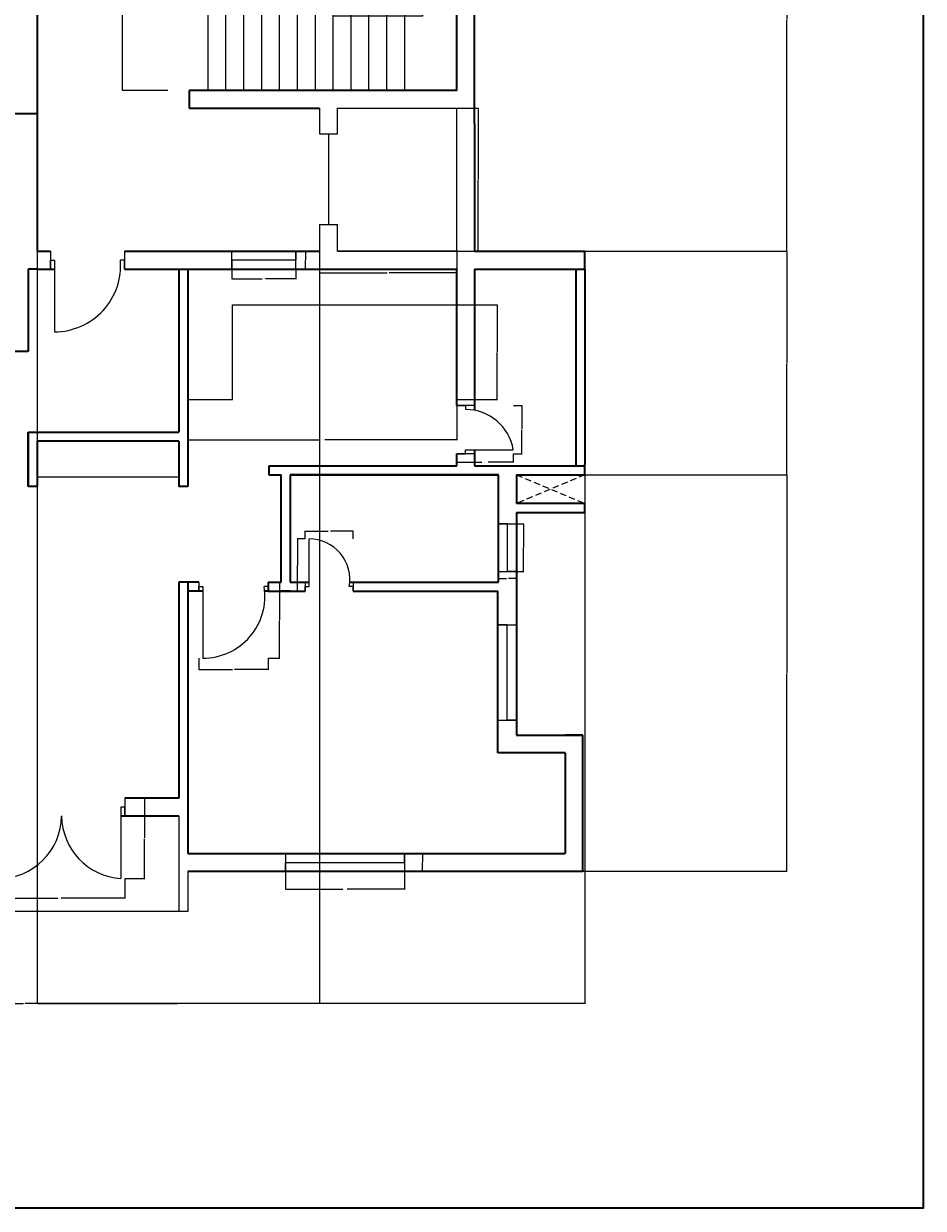
# Model space of a CAD drawing. Units: inches. Extents: x 2296 to 3812, y -1531 to 2564.
# Tile 7 of 10: x 3359 to 3812, y 1124 to 1720. Entities that reach past the tile are written whole.
import ezdxf

# ---------------------------------------------------------------- set-up
doc = ezdxf.new("R2010")
doc.units = ezdxf.units.IN
doc.linetypes.add('HIDDEN2', pattern=[4.7625, 3.175, -1.5875])
for name, color, linetype, lineweight in [('A-ANNO-DIMS', 2, 'Continuous', 18), ('A-ANNO-TTLB', 7, 'Continuous', 35), ('A-DOOR', 3, 'Continuous', 18), ('A-EQPM-ELEV', 7, 'Continuous', 25), ('A-FLOR-CASE', 8, 'Continuous', 18), ('A-FLOR-HRAL', 7, 'Continuous', 25), ('A-FLOR-STRS', 7, 'Continuous', 18), ('A-GLAZ', 4, 'Continuous', 18), ('A-WALL', 7, 'Continuous', 35), ('A-WALL-HIDN', 8, 'HIDDEN2', 18)]:
    doc.layers.add(name, color=color, linetype=linetype, lineweight=lineweight)
doc.styles.get("Standard").update_dxf_attribs({"font": 'arial.ttf'})
doc.dimstyles.get("Standard").update_dxf_attribs({"dimtxt": 0.18, "dimasz": 0.18, "dimexe": 0.18, "dimexo": 0.0625, "dimgap": 0.09, "dimtad": 0, "dimtih": 1, "dimtoh": 1, "dimdec": 4, "dimzin": 0, "dimdsep": 46, "dimtxsty": 'Standard', "dimcen": 0.09, "dimadec": 0, "dimazin": 0, "dimtfac": 1, "dimtdec": 4, "dimtofl": 0, "dimtmove": 0, "dimatfit": 3, "dimfxl": 1, "dimtolj": 1, "dimtzin": 0, "dimarcsym": 0})

# ---------------------------------------------------------------- blocks, each defined once
blk = doc.blocks.new('DOOR-ENTRY-36-S')
for p, q in [((0, 40.5), (0, 31.5)), ((0, 31.5), (0, 36)), ((0, 36), (2, 36)), ((2, 36), (2, 0)), ((37.2, 36), (35.2, 36)), ((37.2, 40.5), (37.2, 31.5)), ((37.2, 31.5), (37.2, 36))]:
    blk.add_line(p, q)
blk.add_arc((2, 33.31), 33.31, 270, 4.6283)
blk = doc.blocks.new('DOOR-BEDROOM-36-SE')
for p, q in [((0, 38.25), (0, 33.75)), ((0, 33.75), (0, 36)), ((0, 36), (2, 36)), ((2, 36), (2, 0)), ((34.88, 36), (32.88, 36))]:
    blk.add_line(p, q)
blk.add_arc((2, 31.24), 31.24, 270, 8.75969)
blk = doc.blocks.new('DOOR-BATH-24-SE')
for p, q in [((2, 2.25), (2, 26.25)), ((0, 4.5), (0, 0)), ((0, 0), (0, 2.25)), ((0, 2.25), (2, 2.25)), ((24.15, 2.25), (22.15, 2.25)), ((24.15, 4.5), (24.15, 0)), ((24.15, 0), (24.15, 2.25))]:
    blk.add_line(p, q)
blk.add_arc((2, 5.79), 20.46, 350.03773, 90)
blk = doc.blocks.new('DOOR-BALCONY-PAIR-S')
for p, q in [((0, 40.5), (0, 31.5)), ((0, 31.5), (0, 36)), ((0, 36), (2, 36)), ((2, 36), (2, 0)), ((65.68, 36), (63.68, 36)), ((63.68, 36), (63.68, 0)), ((65.68, 40.5), (65.68, 31.5)), ((65.68, 31.5), (65.68, 36))]:
    blk.add_line(p, q)
for centre, radius, start, end in [((2, 31.87), 31.87, 270, 359.32793), ((65.8, 31.86), 31.93, 180.64039, 266.18908)]:
    blk.add_arc(centre, radius, start, end)
blk = doc.blocks.new('DOOR-SERVICE-24-SE')
for p, q in [((9, 24.24), (0, 24.24)), ((0, 24.24), (4.5, 24.24)), ((4.5, 24.24), (4.5, 22.24)), ((9, 0), (0, 0)), ((0, 0), (4.5, 0)), ((4.5, 0), (4.5, 2)), ((4.5, 2), (28.5, 2))]:
    blk.add_line(p, q)
blk.add_arc((4.5, -2.11), 24.35, 9.71884, 90)
blk = doc.blocks.new('WIN-24-BATH')
for p, q in [((4.5, 24), (0, 24)), ((0, 24), (9, 24)), ((4.5, 0), (4.5, 24)), ((0, 0), (9, 0)), ((9, 0), (4.5, 0))]:
    blk.add_line(p, q)
blk = doc.blocks.new('WIN-48-BEDROOM-SE')
for p, q in [((4.71, 48), (0, 48)), ((0, 48), (9.41, 48)), ((4.71, 0), (4.71, 48)), ((0, 0), (9.41, 0)), ((9.41, 0), (4.71, 0))]:
    blk.add_line(p, q)
blk = doc.blocks.new('WIN-60-SILL')
for p, q in [((0, 9), (0, 0)), ((60, 4.5), (60, 9)), ((60, 9), (60, 0)), ((0, 0), (0, 4.5)), ((0, 4.5), (60, 4.5))]:
    blk.add_line(p, q)
blk = doc.blocks.new('WIN-32-KITCHEN')
for p, q in [((0, 9), (0, 0)), ((32.18, 4.5), (32.18, 9)), ((32.18, 9), (32.18, 0)), ((0, 0), (0, 4.5)), ((0, 4.5), (32.18, 4.5))]:
    blk.add_line(p, q)
blk = doc.blocks.new('STAIR-DOGLEG')
for p, q in [((20.27, 0), (20.27, 152.06)), ((29.27, 0), (29.27, 152.06)), ((38.27, 0), (38.27, 152.06)), ((47.27, 0), (47.27, 152.06)), ((56.27, 0), (56.27, 152.06)), ((65.27, 0), (65.27, 152.06)), ((74.27, 0), (74.27, 152.06)), ((83.27, 0), (83.27, 152.06)), ((92.27, 0), (92.27, 152.06)), ((101.27, 0), (101.27, 152.06)), ((110.27, 0), (110.27, 152.06)), ((119.27, 0), (119.27, 152.06)), ((0, 107.85), (128.27, 107.85)), ((128.27, 107.85), (128.27, 37.4)), ((20.27, 76.03), (119.27, 76.03)), ((128.27, 37.4), (83.27, 37.4))]:
    blk.add_line(p, q)
blk = doc.blocks.new('COUNTER-KITCHEN-S')
for p, q in [((22.51, 0), (22.51, 47.52)), ((22.51, 47.52), (135.34, 47.52)), ((0, 0), (0, 0)), ((0, 0), (22.51, 0))]:
    blk.add_line(p, q)
blk = doc.blocks.new('LIFT-SHAFT-60x72')
for p, q in [((0, 72), (0, 59.12)), ((9, 72), (69, 72)), ((9, 59.12), (9, 72)), ((69, 0), (69, 72)), ((0, 59.12), (9, 59.12)), ((4.5, 59.12), (4.5, 13.58)), ((0, 13.58), (9, 13.58)), ((0, 13.58), (0, 0)), ((9, 0), (9, 13.58)), ((69, 0), (9, 0)), ((9, 0), (69, 0))]:
    blk.add_line(p, q)
blk = doc.blocks.new('*D49')
at = {"layer": 'A-ANNO-DIMS', "color": 0, "lineweight": -2, "transparency": 16777216}
for p, q in [((3431.99, 1838.66), (3409.07, 1838.66)), ((3409.25, 1838.48), (3409.25, 1762.81)), ((3409.25, 1686.78), (3409.25, 1762.45)), ((3431.99, 1686.6), (3409.07, 1686.6))]:
    blk.add_line(p, q, dxfattribs=at)
at = {"layer": 'A-ANNO-DIMS', "color": 0, "transparency": 16777216}
for points in [[(3409.22, 1838.48), (3409.28, 1838.48), (3409.25, 1838.66)], [(3409.22, 1686.78), (3409.28, 1686.78), (3409.25, 1686.6)]]:
    blk.add_solid(points, dxfattribs=at)
at = {"layer": 'Defpoints', "color": 0, "transparency": 16777216}
for p in [(3409.25, 1838.66), (3432.06, 1838.66), (3432.06, 1686.6)]:
    blk.add_point(p, dxfattribs=at)
at = {"layer": 'A-ANNO-DIMS', "color": 0, "transparency": 16777216, "insert": (3409.25, 1762.63), "char_height": 0.18, "attachment_point": 5}
blk.add_mtext('\\A1;STAIR 152 TYP.', dxfattribs=at)
blk = doc.blocks.new('*D51')
at = {"layer": 'A-ANNO-DIMS', "color": 0, "lineweight": -2, "transparency": 16777216}
for p, q in [((3577.56, 1677.6), (3588.47, 1677.6)), ((3588.29, 1677.42), (3588.29, 1641.78)), ((3588.29, 1605.78), (3588.29, 1641.42)), ((3577.56, 1605.6), (3588.47, 1605.6))]:
    blk.add_line(p, q, dxfattribs=at)
at = {"layer": 'A-ANNO-DIMS', "color": 0, "transparency": 16777216}
for points in [[(3588.26, 1677.42), (3588.32, 1677.42), (3588.29, 1677.6)], [(3588.26, 1605.78), (3588.32, 1605.78), (3588.29, 1605.6)]]:
    blk.add_solid(points, dxfattribs=at)
at = {"layer": 'Defpoints', "color": 0, "transparency": 16777216}
for p in [(3577.49, 1677.6), (3588.29, 1677.6), (3577.49, 1605.6)]:
    blk.add_point(p, dxfattribs=at)
at = {"layer": 'A-ANNO-DIMS', "color": 0, "transparency": 16777216, "insert": (3588.29, 1641.6), "char_height": 0.18, "attachment_point": 5}
blk.add_mtext('\\A1;LIFT 72 TYP.', dxfattribs=at)
blk = doc.blocks.new('*D52')
at = {"layer": 'A-ANNO-DIMS', "color": 0, "lineweight": -2, "transparency": 16777216}
for p, q in [((3508.49, 1605.54), (3508.49, 1594.62)), ((3577.49, 1605.54), (3577.49, 1594.62)), ((3508.67, 1594.8), (3542.47, 1594.8)), ((3577.31, 1594.8), (3543.52, 1594.8))]:
    blk.add_line(p, q, dxfattribs=at)
at = {"layer": 'A-ANNO-DIMS', "color": 0, "transparency": 16777216}
for points in [[(3508.67, 1594.83), (3508.67, 1594.77), (3508.49, 1594.8)], [(3577.31, 1594.83), (3577.31, 1594.77), (3577.49, 1594.8)]]:
    blk.add_solid(points, dxfattribs=at)
at = {"layer": 'Defpoints', "color": 0, "transparency": 16777216}
for p in [(3508.49, 1605.6), (3577.49, 1605.6), (3577.49, 1594.8)]:
    blk.add_point(p, dxfattribs=at)
at = {"layer": 'A-ANNO-DIMS', "color": 0, "transparency": 16777216, "insert": (3542.99, 1594.8), "char_height": 0.18, "attachment_point": 5}
blk.add_mtext('\\A1;69 TYP.', dxfattribs=at)
blk = doc.blocks.new('*D55')
at = {"layer": 'A-ANNO-DIMS', "color": 0, "lineweight": -2, "transparency": 16777216}
for p, q in [((3442.16, 1531.04), (3442.16, 1510.62)), ((3577.49, 1531.04), (3577.49, 1510.62)), ((3442.34, 1510.8), (3508.57, 1510.8)), ((3577.31, 1510.8), (3511.08, 1510.8))]:
    blk.add_line(p, q, dxfattribs=at)
at = {"layer": 'A-ANNO-DIMS', "color": 0, "transparency": 16777216}
for points in [[(3442.34, 1510.83), (3442.34, 1510.77), (3442.16, 1510.8)], [(3577.31, 1510.83), (3577.31, 1510.77), (3577.49, 1510.8)]]:
    blk.add_solid(points, dxfattribs=at)
at = {"layer": 'Defpoints', "color": 0, "transparency": 16777216}
for p in [(3442.16, 1531.1), (3577.49, 1531.1), (3577.49, 1510.8)]:
    blk.add_point(p, dxfattribs=at)
at = {"layer": 'A-ANNO-DIMS', "color": 0, "transparency": 16777216, "insert": (3509.83, 1510.8), "char_height": 0.18, "attachment_point": 5}
blk.add_mtext('\\A1;COUNTER 135 TYP.', dxfattribs=at)
blk = doc.blocks.new('*D56')
at = {"layer": 'A-ANNO-DIMS', "color": 0, "lineweight": -2, "transparency": 16777216}
for p, q in [((3577.56, 1578.62), (3597.97, 1578.62)), ((3597.79, 1578.44), (3597.79, 1555.04)), ((3597.79, 1531.28), (3597.79, 1554.68)), ((3577.56, 1531.1), (3597.97, 1531.1))]:
    blk.add_line(p, q, dxfattribs=at)
at = {"layer": 'A-ANNO-DIMS', "color": 0, "transparency": 16777216}
for points in [[(3597.76, 1578.44), (3597.82, 1578.44), (3597.79, 1578.62)], [(3597.76, 1531.28), (3597.82, 1531.28), (3597.79, 1531.1)]]:
    blk.add_solid(points, dxfattribs=at)
at = {"layer": 'Defpoints', "color": 0, "transparency": 16777216}
for p in [(3577.49, 1578.62), (3597.79, 1578.62), (3577.49, 1531.1)]:
    blk.add_point(p, dxfattribs=at)
at = {"layer": 'A-ANNO-DIMS', "color": 0, "transparency": 16777216, "insert": (3597.79, 1554.86), "char_height": 0.18, "attachment_point": 5}
blk.add_mtext('\\A1;48 TYP.', dxfattribs=at)
blk = doc.blocks.new('*D79')
at = {"layer": 'A-ANNO-DIMS', "color": 0, "lineweight": -2, "transparency": 16777216}
for p, q in [((3482.65, 1439.1), (3488.51, 1439.1)), ((3488.33, 1438.92), (3488.33, 1420.16)), ((3488.33, 1401.03), (3488.33, 1419.79)), ((3482.65, 1400.85), (3488.51, 1400.85))]:
    blk.add_line(p, q, dxfattribs=at)
at = {"layer": 'A-ANNO-DIMS', "color": 0, "transparency": 16777216}
for points in [[(3488.3, 1438.92), (3488.36, 1438.92), (3488.33, 1439.1)], [(3488.3, 1401.03), (3488.36, 1401.03), (3488.33, 1400.85)]]:
    blk.add_solid(points, dxfattribs=at)
at = {"layer": 'Defpoints', "color": 0, "transparency": 16777216}
for p in [(3482.59, 1439.1), (3488.33, 1439.1), (3482.59, 1400.85)]:
    blk.add_point(p, dxfattribs=at)
at = {"layer": 'A-ANNO-DIMS', "color": 0, "transparency": 16777216, "insert": (3488.33, 1419.98), "char_height": 0.18, "attachment_point": 5}
blk.add_mtext('\\A1;DOOR 38 TYP.', dxfattribs=at)
blk = doc.blocks.new('*D80')
at = {"layer": 'A-ANNO-DIMS', "color": 0, "lineweight": -2, "transparency": 16777216}
for p, q in [((3447.71, 1400.79), (3447.71, 1394.93)), ((3447.89, 1395.11), (3464.63, 1395.11)), ((3482.41, 1395.11), (3465.68, 1395.11)), ((3482.59, 1400.79), (3482.59, 1394.93))]:
    blk.add_line(p, q, dxfattribs=at)
at = {"layer": 'A-ANNO-DIMS', "color": 0, "transparency": 16777216}
for points in [[(3447.89, 1395.14), (3447.89, 1395.08), (3447.71, 1395.11)], [(3482.41, 1395.14), (3482.41, 1395.08), (3482.59, 1395.11)]]:
    blk.add_solid(points, dxfattribs=at)
at = {"layer": 'Defpoints', "color": 0, "transparency": 16777216}
for p in [(3447.71, 1400.85), (3482.59, 1400.85), (3482.59, 1395.11)]:
    blk.add_point(p, dxfattribs=at)
at = {"layer": 'A-ANNO-DIMS', "color": 0, "transparency": 16777216, "insert": (3465.15, 1395.11), "char_height": 0.18, "attachment_point": 5}
blk.add_mtext('\\A1;35 TYP.', dxfattribs=at)
blk = doc.blocks.new('*D81')
at = {"layer": 'A-ANNO-DIMS', "color": 0, "lineweight": -2, "transparency": 16777216}
for p, q in [((3501.21, 1460.85), (3497.15, 1460.85)), ((3497.33, 1460.67), (3497.33, 1447.91)), ((3497.33, 1434.78), (3497.33, 1447.54)), ((3501.21, 1434.6), (3497.15, 1434.6))]:
    blk.add_line(p, q, dxfattribs=at)
at = {"layer": 'A-ANNO-DIMS', "color": 0, "transparency": 16777216}
for points in [[(3497.3, 1460.67), (3497.36, 1460.67), (3497.33, 1460.85)], [(3497.3, 1434.78), (3497.36, 1434.78), (3497.33, 1434.6)]]:
    blk.add_solid(points, dxfattribs=at)
at = {"layer": 'Defpoints', "color": 0, "transparency": 16777216}
for p in [(3497.33, 1460.85), (3501.27, 1460.85), (3501.27, 1434.6)]:
    blk.add_point(p, dxfattribs=at)
at = {"layer": 'A-ANNO-DIMS', "color": 0, "transparency": 16777216, "insert": (3497.33, 1447.73), "char_height": 0.18, "attachment_point": 5}
blk.add_mtext('\\A1;BATH DOOR 26 TYP.', dxfattribs=at)
blk = doc.blocks.new('*D82')
at = {"layer": 'A-ANNO-DIMS', "color": 0, "lineweight": -2, "transparency": 16777216}
for p, q in [((3501.27, 1460.91), (3501.27, 1464.97)), ((3501.45, 1464.79), (3512.82, 1464.79)), ((3525.24, 1464.79), (3513.88, 1464.79)), ((3525.42, 1460.91), (3525.42, 1464.97))]:
    blk.add_line(p, q, dxfattribs=at)
at = {"layer": 'A-ANNO-DIMS', "color": 0, "transparency": 16777216}
for points in [[(3501.45, 1464.82), (3501.45, 1464.76), (3501.27, 1464.79)], [(3525.24, 1464.82), (3525.24, 1464.76), (3525.42, 1464.79)]]:
    blk.add_solid(points, dxfattribs=at)
at = {"layer": 'Defpoints', "color": 0, "transparency": 16777216}
for p in [(3501.27, 1460.85), (3525.42, 1464.79), (3525.42, 1460.85)]:
    blk.add_point(p, dxfattribs=at)
at = {"layer": 'A-ANNO-DIMS', "color": 0, "transparency": 16777216, "insert": (3513.35, 1464.79), "char_height": 0.18, "attachment_point": 5}
blk.add_mtext('\\A1;24 TYP.', dxfattribs=at)
blk = doc.blocks.new('*D87')
at = {"layer": 'A-ANNO-DIMS', "color": 0, "lineweight": -2, "transparency": 16777216}
for p, q in [((3344.71, 1289.87), (3344.71, 1279.9)), ((3410.39, 1289.87), (3410.39, 1279.9)), ((3344.89, 1280.08), (3376.7, 1280.08)), ((3410.21, 1280.08), (3378.4, 1280.08))]:
    blk.add_line(p, q, dxfattribs=at)
at = {"layer": 'A-ANNO-DIMS', "color": 0, "transparency": 16777216}
for points in [[(3344.89, 1280.11), (3344.89, 1280.05), (3344.71, 1280.08)], [(3410.21, 1280.11), (3410.21, 1280.05), (3410.39, 1280.08)]]:
    blk.add_solid(points, dxfattribs=at)
at = {"layer": 'Defpoints', "color": 0, "transparency": 16777216}
for p in [(3344.71, 1289.93), (3410.39, 1289.93), (3410.39, 1280.08)]:
    blk.add_point(p, dxfattribs=at)
at = {"layer": 'A-ANNO-DIMS', "color": 0, "transparency": 16777216, "insert": (3377.55, 1280.08), "char_height": 0.18, "attachment_point": 5}
blk.add_mtext('\\A1;PAIR 66 TYP.', dxfattribs=at)
blk = doc.blocks.new('*D88')
at = {"layer": 'A-ANNO-DIMS', "color": 0, "lineweight": -2, "transparency": 16777216}
for p, q in [((3410.45, 1330.43), (3420.42, 1330.43)), ((3420.24, 1330.25), (3420.24, 1310.36)), ((3420.24, 1290.11), (3420.24, 1310)), ((3410.45, 1289.93), (3420.42, 1289.93))]:
    blk.add_line(p, q, dxfattribs=at)
at = {"layer": 'A-ANNO-DIMS', "color": 0, "transparency": 16777216}
for points in [[(3420.21, 1330.25), (3420.27, 1330.25), (3420.24, 1330.43)], [(3420.21, 1290.11), (3420.27, 1290.11), (3420.24, 1289.93)]]:
    blk.add_solid(points, dxfattribs=at)
at = {"layer": 'Defpoints', "color": 0, "transparency": 16777216}
for p in [(3410.39, 1330.43), (3420.24, 1330.43), (3410.39, 1289.93)]:
    blk.add_point(p, dxfattribs=at)
at = {"layer": 'A-ANNO-DIMS', "color": 0, "transparency": 16777216, "insert": (3420.24, 1310.18), "char_height": 0.18, "attachment_point": 5}
blk.add_mtext('\\A1;41 TYP.', dxfattribs=at)
blk = doc.blocks.new('*D91')
at = {"layer": 'A-ANNO-DIMS', "color": 0, "lineweight": -2, "transparency": 16777216}
for p, q in [((3577.49, 1503.68), (3577.49, 1499.29)), ((3605.99, 1503.68), (3605.99, 1499.29)), ((3577.67, 1499.47), (3590.22, 1499.47)), ((3605.81, 1499.47), (3593.27, 1499.47))]:
    blk.add_line(p, q, dxfattribs=at)
at = {"layer": 'A-ANNO-DIMS', "color": 0, "transparency": 16777216}
for points in [[(3577.67, 1499.5), (3577.67, 1499.44), (3577.49, 1499.47)], [(3605.81, 1499.5), (3605.81, 1499.44), (3605.99, 1499.47)]]:
    blk.add_solid(points, dxfattribs=at)
at = {"layer": 'Defpoints', "color": 0, "transparency": 16777216}
for p in [(3577.49, 1503.74), (3605.99, 1503.74), (3605.99, 1499.47)]:
    blk.add_point(p, dxfattribs=at)
at = {"layer": 'A-ANNO-DIMS', "color": 0, "transparency": 16777216, "insert": (3591.74, 1499.47), "char_height": 0.18, "attachment_point": 5}
blk.add_mtext('\\A1;SERVICE DOOR 29 TYP.', dxfattribs=at)
blk = doc.blocks.new('*D92')
at = {"layer": 'A-ANNO-DIMS', "color": 0, "lineweight": -2, "transparency": 16777216}
for p, q in [((3606.06, 1527.98), (3610.45, 1527.98)), ((3610.27, 1527.8), (3610.27, 1516.04)), ((3610.27, 1503.92), (3610.27, 1515.68)), ((3606.06, 1503.74), (3610.45, 1503.74))]:
    blk.add_line(p, q, dxfattribs=at)
at = {"layer": 'A-ANNO-DIMS', "color": 0, "transparency": 16777216}
for points in [[(3610.24, 1527.8), (3610.3, 1527.8), (3610.27, 1527.98)], [(3610.24, 1503.92), (3610.3, 1503.92), (3610.27, 1503.74)]]:
    blk.add_solid(points, dxfattribs=at)
at = {"layer": 'Defpoints', "color": 0, "transparency": 16777216}
for p in [(3605.99, 1527.98), (3610.27, 1527.98), (3605.99, 1503.74)]:
    blk.add_point(p, dxfattribs=at)
at = {"layer": 'A-ANNO-DIMS', "color": 0, "transparency": 16777216, "insert": (3610.27, 1515.86), "char_height": 0.18, "attachment_point": 5}
blk.add_mtext('\\A1;24 TYP.', dxfattribs=at)
blk = doc.blocks.new('*D93')
at = {"layer": 'A-ANNO-DIMS', "color": 0, "lineweight": -2, "transparency": 16777216}
for p, q in [((3607.63, 1468.51), (3611.35, 1468.51)), ((3611.17, 1468.33), (3611.17, 1456.7)), ((3611.17, 1444.69), (3611.17, 1456.33)), ((3607.63, 1444.51), (3611.35, 1444.51))]:
    blk.add_line(p, q, dxfattribs=at)
at = {"layer": 'A-ANNO-DIMS', "color": 0, "transparency": 16777216}
for points in [[(3611.14, 1468.33), (3611.2, 1468.33), (3611.17, 1468.51)], [(3611.14, 1444.69), (3611.2, 1444.69), (3611.17, 1444.51)]]:
    blk.add_solid(points, dxfattribs=at)
at = {"layer": 'Defpoints', "color": 0, "transparency": 16777216}
for p in [(3607.57, 1468.51), (3611.17, 1468.51), (3607.57, 1444.51)]:
    blk.add_point(p, dxfattribs=at)
at = {"layer": 'A-ANNO-DIMS', "color": 0, "transparency": 16777216, "insert": (3611.17, 1456.51), "char_height": 0.18, "attachment_point": 5}
blk.add_mtext('\\A1;WINDOW 24 TYP.', dxfattribs=at)
blk = doc.blocks.new('*D94')
at = {"layer": 'A-ANNO-DIMS', "color": 0, "lineweight": -2, "transparency": 16777216}
for p, q in [((3598.57, 1444.45), (3598.57, 1440.73)), ((3607.57, 1444.45), (3607.57, 1440.73)), ((3598.75, 1440.91), (3602.61, 1440.91)), ((3607.39, 1440.91), (3603.53, 1440.91))]:
    blk.add_line(p, q, dxfattribs=at)
at = {"layer": 'A-ANNO-DIMS', "color": 0, "transparency": 16777216}
for points in [[(3598.75, 1440.94), (3598.75, 1440.88), (3598.57, 1440.91)], [(3607.39, 1440.94), (3607.39, 1440.88), (3607.57, 1440.91)]]:
    blk.add_solid(points, dxfattribs=at)
at = {"layer": 'Defpoints', "color": 0, "transparency": 16777216}
for p in [(3598.57, 1444.51), (3607.57, 1444.51), (3607.57, 1440.91)]:
    blk.add_point(p, dxfattribs=at)
at = {"layer": 'A-ANNO-DIMS', "color": 0, "transparency": 16777216, "insert": (3603.07, 1440.91), "char_height": 0.18, "attachment_point": 5}
blk.add_mtext('\\A1;9 TYP.', dxfattribs=at)
blk = doc.blocks.new('*D97')
at = {"layer": 'A-ANNO-DIMS', "color": 0, "lineweight": -2, "transparency": 16777216}
for p, q in [((3491.22, 1293.54), (3491.22, 1284.42)), ((3551.22, 1293.54), (3551.22, 1284.42)), ((3491.4, 1284.6), (3520.11, 1284.6)), ((3551.04, 1284.6), (3522.34, 1284.6))]:
    blk.add_line(p, q, dxfattribs=at)
at = {"layer": 'A-ANNO-DIMS', "color": 0, "transparency": 16777216}
for points in [[(3491.4, 1284.63), (3491.4, 1284.57), (3491.22, 1284.6)], [(3551.04, 1284.63), (3551.04, 1284.57), (3551.22, 1284.6)]]:
    blk.add_solid(points, dxfattribs=at)
at = {"layer": 'Defpoints', "color": 0, "transparency": 16777216}
for p in [(3491.22, 1293.6), (3551.22, 1293.6), (3551.22, 1284.6)]:
    blk.add_point(p, dxfattribs=at)
at = {"layer": 'A-ANNO-DIMS', "color": 0, "transparency": 16777216, "insert": (3521.22, 1284.6), "char_height": 0.18, "attachment_point": 5}
blk.add_mtext('\\A1;WINDOW 60 TYP.', dxfattribs=at)
blk = doc.blocks.new('*D98')
at = {"layer": 'A-ANNO-DIMS', "color": 0, "lineweight": -2, "transparency": 16777216}
for p, q in [((3551.29, 1302.6), (3560.4, 1302.6)), ((3560.22, 1302.42), (3560.22, 1298.28)), ((3560.22, 1293.78), (3560.22, 1297.92)), ((3551.29, 1293.6), (3560.4, 1293.6))]:
    blk.add_line(p, q, dxfattribs=at)
at = {"layer": 'A-ANNO-DIMS', "color": 0, "transparency": 16777216}
for points in [[(3560.19, 1302.42), (3560.25, 1302.42), (3560.22, 1302.6)], [(3560.19, 1293.78), (3560.25, 1293.78), (3560.22, 1293.6)]]:
    blk.add_solid(points, dxfattribs=at)
at = {"layer": 'Defpoints', "color": 0, "transparency": 16777216}
for p in [(3551.22, 1302.6), (3560.22, 1302.6), (3551.22, 1293.6)]:
    blk.add_point(p, dxfattribs=at)
at = {"layer": 'A-ANNO-DIMS', "color": 0, "transparency": 16777216, "insert": (3560.22, 1298.1), "char_height": 0.18, "attachment_point": 5}
blk.add_mtext('\\A1;9 TYP.', dxfattribs=at)
blk = doc.blocks.new('*D115')
at = {"layer": 'A-ANNO-DIMS', "color": 0, "lineweight": -2, "transparency": 16777216}
for p, q in [((3464.36, 1596.54), (3464.36, 1591.59)), ((3464.54, 1591.77), (3479.6, 1591.77)), ((3496.35, 1591.77), (3481.29, 1591.77)), ((3496.53, 1596.54), (3496.53, 1591.59))]:
    blk.add_line(p, q, dxfattribs=at)
at = {"layer": 'A-ANNO-DIMS', "color": 0, "transparency": 16777216}
for points in [[(3464.54, 1591.8), (3464.54, 1591.74), (3464.36, 1591.77)], [(3496.35, 1591.8), (3496.35, 1591.74), (3496.53, 1591.77)]]:
    blk.add_solid(points, dxfattribs=at)
at = {"layer": 'Defpoints', "color": 0, "transparency": 16777216}
for p in [(3464.36, 1596.6), (3464.36, 1591.77), (3496.53, 1596.6)]:
    blk.add_point(p, dxfattribs=at)
at = {"layer": 'A-ANNO-DIMS', "color": 0, "transparency": 16777216, "insert": (3480.45, 1591.77), "char_height": 0.18, "attachment_point": 5}
blk.add_mtext('\\A1;WIN. 32 TYP.', dxfattribs=at)
blk = doc.blocks.new('*D116')
at = {"layer": 'A-ANNO-DIMS', "color": 0, "lineweight": -2, "transparency": 16777216}
for p, q in [((3496.6, 1605.6), (3501.54, 1605.6)), ((3501.36, 1605.42), (3501.36, 1601.28)), ((3501.36, 1596.78), (3501.36, 1600.92)), ((3496.6, 1596.6), (3501.54, 1596.6))]:
    blk.add_line(p, q, dxfattribs=at)
at = {"layer": 'A-ANNO-DIMS', "color": 0, "transparency": 16777216}
for points in [[(3501.33, 1605.42), (3501.39, 1605.42), (3501.36, 1605.6)], [(3501.33, 1596.78), (3501.39, 1596.78), (3501.36, 1596.6)]]:
    blk.add_solid(points, dxfattribs=at)
at = {"layer": 'Defpoints', "color": 0, "transparency": 16777216}
for p in [(3496.53, 1605.6), (3496.53, 1596.6), (3501.36, 1596.6)]:
    blk.add_point(p, dxfattribs=at)
at = {"layer": 'A-ANNO-DIMS', "color": 0, "transparency": 16777216, "insert": (3501.36, 1601.1), "char_height": 0.18, "attachment_point": 5}
blk.add_mtext('\\A1;9 TYP.', dxfattribs=at)
blk = doc.blocks.new('*D129')
at = {"layer": 'A-ANNO-DIMS', "color": 0, "lineweight": -2, "transparency": 16777216}
for p, q in [((3641.99, 1498.34), (3641.99, 1226.9)), ((3077.66, 1427.77), (3077.66, 1226.9)), ((3077.84, 1227.08), (3359.43, 1227.08)), ((3641.81, 1227.08), (3360.22, 1227.08))]:
    blk.add_line(p, q, dxfattribs=at)
at = {"layer": 'A-ANNO-DIMS', "color": 0, "transparency": 16777216}
for points in [[(3077.84, 1227.11), (3077.84, 1227.05), (3077.66, 1227.08)], [(3641.81, 1227.11), (3641.81, 1227.05), (3641.99, 1227.08)]]:
    blk.add_solid(points, dxfattribs=at)
at = {"layer": 'Defpoints', "color": 0, "transparency": 16777216}
for p in [(3641.99, 1498.4), (3077.66, 1427.84), (3641.99, 1227.08)]:
    blk.add_point(p, dxfattribs=at)
at = {"layer": 'A-ANNO-DIMS', "color": 0, "transparency": 16777216, "insert": (3359.83, 1227.08), "char_height": 0.18, "attachment_point": 5}
blk.add_mtext('\\A1;564.3', dxfattribs=at)
blk = doc.blocks.new('*D134')
at = {"layer": 'A-ANNO-DIMS', "color": 0, "lineweight": -2, "transparency": 16777216}
for p, q in [((3642.06, 1493.1), (3743.91, 1493.1)), ((3743.73, 1492.92), (3743.73, 1393.53)), ((3743.73, 1293.78), (3743.73, 1393.17)), ((3641.1, 1293.6), (3743.91, 1293.6))]:
    blk.add_line(p, q, dxfattribs=at)
at = {"layer": 'A-ANNO-DIMS', "color": 0, "transparency": 16777216}
for points in [[(3743.7, 1492.92), (3743.76, 1492.92), (3743.73, 1493.1)], [(3743.7, 1293.78), (3743.76, 1293.78), (3743.73, 1293.6)]]:
    blk.add_solid(points, dxfattribs=at)
at = {"layer": 'Defpoints', "color": 0, "transparency": 16777216}
for p in [(3641.99, 1493.1), (3743.73, 1493.1), (3641.04, 1293.6)]:
    blk.add_point(p, dxfattribs=at)
at = {"layer": 'A-ANNO-DIMS', "color": 0, "transparency": 16777216, "insert": (3743.73, 1393.35), "char_height": 0.18, "attachment_point": 5}
blk.add_mtext('\\A1;199.5', dxfattribs=at)
blk = doc.blocks.new('*D135')
at = {"layer": 'A-ANNO-DIMS', "color": 0, "lineweight": -2, "transparency": 16777216}
for p, q in [((3642.06, 1605.6), (3743.91, 1605.6)), ((3743.73, 1605.42), (3743.73, 1549.53)), ((3743.73, 1493.28), (3743.73, 1549.17)), ((3642.06, 1493.1), (3743.91, 1493.1))]:
    blk.add_line(p, q, dxfattribs=at)
at = {"layer": 'A-ANNO-DIMS', "color": 0, "transparency": 16777216}
for points in [[(3743.7, 1605.42), (3743.76, 1605.42), (3743.73, 1605.6)], [(3743.7, 1493.28), (3743.76, 1493.28), (3743.73, 1493.1)]]:
    blk.add_solid(points, dxfattribs=at)
at = {"layer": 'Defpoints', "color": 0, "transparency": 16777216}
for p in [(3641.99, 1605.6), (3743.73, 1605.6), (3641.99, 1493.1)]:
    blk.add_point(p, dxfattribs=at)
at = {"layer": 'A-ANNO-DIMS', "color": 0, "transparency": 16777216, "insert": (3743.73, 1549.35), "char_height": 0.18, "attachment_point": 5}
blk.add_mtext('\\A1;112.5', dxfattribs=at)
blk = doc.blocks.new('*D136')
at = {"layer": 'A-ANNO-DIMS', "color": 0, "lineweight": -2, "transparency": 16777216}
for p, q in [((3633.38, 1838.66), (3743.91, 1838.66)), ((3743.73, 1838.48), (3743.73, 1722.31)), ((3743.73, 1605.78), (3743.73, 1721.95)), ((3642.06, 1605.6), (3743.91, 1605.6))]:
    blk.add_line(p, q, dxfattribs=at)
at = {"layer": 'A-ANNO-DIMS', "color": 0, "transparency": 16777216}
for points in [[(3743.7, 1838.48), (3743.76, 1838.48), (3743.73, 1838.66)], [(3743.7, 1605.78), (3743.76, 1605.78), (3743.73, 1605.6)]]:
    blk.add_solid(points, dxfattribs=at)
at = {"layer": 'Defpoints', "color": 0, "transparency": 16777216}
for p in [(3633.32, 1838.66), (3743.73, 1838.66), (3641.99, 1605.6)]:
    blk.add_point(p, dxfattribs=at)
at = {"layer": 'A-ANNO-DIMS', "color": 0, "transparency": 16777216, "insert": (3743.73, 1722.13), "char_height": 0.18, "attachment_point": 5}
blk.add_mtext('\\A1;233.06', dxfattribs=at)
blk = doc.blocks.new('*D139')
at = {"layer": 'A-ANNO-DIMS', "color": 0, "lineweight": -2, "transparency": 16777216}
for p, q in [((3366.26, 1605.54), (3366.26, 1226.9)), ((3508.49, 1605.54), (3508.49, 1226.9)), ((3366.44, 1227.08), (3436.92, 1227.08)), ((3508.31, 1227.08), (3437.83, 1227.08))]:
    blk.add_line(p, q, dxfattribs=at)
at = {"layer": 'A-ANNO-DIMS', "color": 0, "transparency": 16777216}
for points in [[(3366.44, 1227.11), (3366.44, 1227.05), (3366.26, 1227.08)], [(3508.31, 1227.11), (3508.31, 1227.05), (3508.49, 1227.08)]]:
    blk.add_solid(points, dxfattribs=at)
at = {"layer": 'Defpoints', "color": 0, "transparency": 16777216}
for p in [(3366.26, 1605.6), (3508.49, 1605.6), (3508.49, 1227.08)]:
    blk.add_point(p, dxfattribs=at)
at = {"layer": 'A-ANNO-DIMS', "color": 0, "transparency": 16777216, "insert": (3437.38, 1227.08), "char_height": 0.18, "attachment_point": 5}
blk.add_mtext('\\A1;142.23', dxfattribs=at)

msp = doc.modelspace()

# ---------------------------------------------------------------- linework, layer by layer
at = {"layer": 'A-ANNO-TTLB'}
msp.add_lwpolyline([(2296.1257, 2564.2989), (3812.4193, 2564.2989), (3812.4193, 1124.0028), (2296.1257, 1124.0028)], close=True, dxfattribs=at)
at = {"layer": 'A-FLOR-CASE'}
msp.add_line((3366.2116, 1492.0877), (3437.6588, 1492.0877), dxfattribs=at)
at = {"layer": 'A-FLOR-HRAL'}
for p, q in [((3437.6588, 1321.434), (3437.6588, 1302.6012)), ((3437.6588, 1321.434), (3437.6588, 1273.434)), ((3437.6588, 1302.6012), (3437.6588, 1273.434)), ((3442.1588, 1293.6012), (3442.1588, 1273.434)), ((3437.6588, 1273.434), (3323.8418, 1273.434)), ((3442.1588, 1273.434), (3437.6588, 1273.434))]:
    msp.add_line(p, q, dxfattribs=at)
at = {"layer": 'A-WALL'}
for p, q in [((3577.4944, 1686.6012), (3577.4944, 1838.6578)), ((3586.1588, 1838.6578), (3586.4944, 1605.6012)), ((3366.2648, 1780.1578), (3366.2648, 1674.9485)), ((3508.4944, 1686.6012), (3442.7516, 1686.6012)), ((3442.7516, 1686.6012), (3442.7516, 1677.6012)), ((3517.4944, 1686.6012), (3508.4944, 1686.6012)), ((3577.4944, 1686.6012), (3517.4944, 1686.6012)), ((3442.7516, 1677.6012), (3508.4944, 1677.6012)), ((3291.4894, 1674.9485), (3366.2648, 1674.9485)), ((3366.2648, 1674.9485), (3366.2648, 1605.6012)), ((3366.2648, 1605.6012), (3372.9833, 1605.6012)), ((3410.1867, 1605.6012), (3508.4944, 1605.6012)), ((3586.4944, 1605.6012), (3641.9944, 1605.6012)), ((3641.9944, 1596.6012), (3641.9944, 1605.6012)), ((3366.2648, 1596.6012), (3361.7116, 1596.6012)), ((3361.7116, 1596.6012), (3361.7116, 1555.1578)), ((3366.2648, 1596.6012), (3374.9833, 1596.6012)), ((3410.1867, 1596.6012), (3577.4944, 1596.6012)), ((3437.6588, 1596.6012), (3437.6588, 1514.5213)), ((3442.1588, 1596.6012), (3442.1588, 1487.3045)), ((3442.1588, 1596.6012), (3571.1588, 1596.6012)), ((3577.4944, 1527.9833), (3577.4944, 1596.6012)), ((3586.4944, 1596.6012), (3637.4944, 1596.6012)), ((3586.4944, 1596.6012), (3586.4944, 1525.5639)), ((3586.4944, 1596.6012), (3637.4944, 1596.6012)), ((3637.4944, 1596.6012), (3637.4944, 1497.6012)), ((3637.4944, 1596.6012), (3641.9944, 1596.6012)), ((3641.9944, 1596.6012), (3641.9944, 1498.4048)), ((3361.7116, 1555.1578), (3286.9894, 1555.1578)), ((3577.4944, 1538.1945), (3577.4944, 1538.1945)), ((3361.7116, 1514.5213), (3361.7116, 1487.3045)), ((3361.7116, 1487.3045), (3361.7116, 1514.5213)), ((3361.7116, 1514.5213), (3437.6588, 1514.5213)), ((3437.6588, 1510.0213), (3366.2116, 1510.0213)), ((3366.2116, 1510.0213), (3366.2116, 1487.3045)), ((3437.6588, 1510.0213), (3437.6588, 1487.3045)), ((3577.4944, 1497.6012), (3577.4944, 1503.7443)), ((3586.4944, 1505.7443), (3586.4944, 1497.6012)), ((3482.9535, 1497.6012), (3577.4944, 1497.6012)), ((3482.9535, 1497.6012), (3482.9535, 1493.1012)), ((3586.4944, 1497.6012), (3637.4944, 1497.6012)), ((3637.4944, 1497.6012), (3641.9944, 1497.6012)), ((3641.9944, 1493.1012), (3641.9944, 1498.4048)), ((3482.9535, 1493.1012), (3489.069, 1493.1012)), ((3489.069, 1439.1012), (3489.069, 1493.1012)), ((3493.569, 1493.1012), (3598.569, 1493.1012)), ((3598.569, 1493.1012), (3493.569, 1493.1012)), ((3493.569, 1493.1012), (3493.569, 1439.1012)), ((3598.569, 1439.1012), (3598.569, 1493.1012)), ((3607.569, 1493.1012), (3637.4944, 1493.1012)), ((3607.569, 1493.1012), (3607.569, 1478.7391)), ((3637.4944, 1493.1012), (3641.9944, 1493.1012)), ((3366.2116, 1487.3045), (3361.7116, 1487.3045)), ((3442.1588, 1487.3045), (3437.6588, 1487.3045)), ((3641.9944, 1478.7391), (3607.569, 1478.7391)), ((3641.9944, 1474.2391), (3641.9944, 1478.7391)), ((3607.569, 1474.2391), (3607.569, 1439.1012)), ((3607.569, 1474.2391), (3641.9944, 1474.2391)), ((3437.6588, 1439.1012), (3437.6588, 1330.434)), ((3447.7145, 1439.1012), (3437.6588, 1439.1012)), ((3442.1588, 1439.1012), (3442.1588, 1302.6012)), ((3482.5922, 1439.1012), (3489.069, 1439.1012)), ((3482.5922, 1439.1012), (3482.5922, 1434.6012)), ((3493.569, 1439.1012), (3503.2701, 1439.1012)), ((3523.6898, 1439.1012), (3598.569, 1439.1012)), ((3607.569, 1439.1012), (3607.569, 1362.1926)), ((3449.7145, 1434.6012), (3442.1588, 1434.6012)), ((3482.5922, 1434.6012), (3480.8558, 1434.6012)), ((3482.5922, 1434.6012), (3501.2701, 1434.6012)), ((3493.569, 1434.6012), (3489.069, 1434.6012)), ((3525.422, 1434.6012), (3598.1588, 1434.6012)), ((3598.1588, 1353.1926), (3598.1588, 1434.6012)), ((3607.569, 1362.1926), (3641.0372, 1362.1926)), ((3641.0372, 1362.1926), (3632.0372, 1362.1926)), ((3641.0372, 1293.6012), (3641.0372, 1362.1926)), ((3632.0372, 1353.1926), (3598.1588, 1353.1926)), ((3632.0372, 1353.1926), (3632.0372, 1302.6012)), ((3437.6588, 1330.434), (3410.3896, 1330.434)), ((3408.3896, 1321.434), (3437.6588, 1321.434)), ((3442.1588, 1302.6012), (3632.0372, 1302.6012)), ((3442.1588, 1302.6012), (3598.1588, 1302.6012)), ((3442.1588, 1293.6012), (3637.4944, 1293.6012)), ((3637.4944, 1293.6012), (3641.0372, 1293.6012))]:
    msp.add_line(p, q, dxfattribs=at)
at = {"layer": 'A-WALL-HIDN'}
for p, q in [((3641.9944, 1493.1012), (3607.569, 1478.7391)), ((3607.569, 1493.1012), (3641.9944, 1478.7391))]:
    msp.add_line(p, q, dxfattribs=at)

# ---------------------------------------------------------------- block references
at = {"layer": 'A-DOOR'}
for name, p in [('DOOR-ENTRY-36-S', (3372.9834, 1565.101)), ('DOOR-SERVICE-24-SE', (3577.4944, 1503.744)), ('DOOR-BATH-24-SE', (3501.2704, 1434.601)), ('DOOR-BEDROOM-36-SE', (3447.7144, 1400.851)), ('DOOR-BALCONY-PAIR-S', (3344.7144, 1289.934))]:
    msp.add_blockref(name, p, dxfattribs=at)
at = {"layer": 'A-EQPM-ELEV'}
msp.add_blockref('LIFT-SHAFT-60x72', (3508.4944, 1605.601), dxfattribs=at)
at = {"layer": 'A-FLOR-CASE'}
msp.add_blockref('COUNTER-KITCHEN-S', (3442.1584, 1531.098), dxfattribs=at)
at = {"layer": 'A-FLOR-STRS'}
msp.add_blockref('STAIR-DOGLEG', (3432.0574, 1686.601), dxfattribs=at)
at = {"layer": 'A-GLAZ', "rotation": 180}
msp.add_blockref('WIN-32-KITCHEN', (3496.5342, 1605.6014), dxfattribs=at)
at = {"layer": 'A-GLAZ'}
for name, p in [('WIN-24-BATH', (3598.5688, 1444.5142)), ('WIN-48-BEDROOM-SE', (3598.1584, 1369.691)), ('WIN-60-SILL', (3491.2244, 1293.601))]:
    msp.add_blockref(name, p, dxfattribs=at)

# ---------------------------------------------------------------- dimensions: what is measured, and where the dimension line sits
at = {"layer": 'A-ANNO-DIMS'}
for base, p1, p2, angle, text, picture, middle in [((3409.2489, 1838.6578), (3432.0574, 1686.6012), (3432.0574, 1838.6578), 90, 'STAIR <> TYP.', '*D49', (3409.2489, 1762.6295)), ((3588.2944, 1677.6012), (3577.4944, 1605.6012), (3577.4944, 1677.6012), 90, 'LIFT <> TYP.', '*D51', (3588.2944, 1641.6012)), ((3501.3603, 1596.6012), (3496.5339, 1605.6012), (3496.5339, 1596.6012), 270, '<> TYP.', '*D116', (3501.3603, 1601.1012)), ((3464.3578, 1591.7748), (3496.5339, 1596.6012), (3464.3578, 1596.6012), 180, 'WIN. <> TYP.', '*D115', (3480.4458, 1591.7748)), ((3597.7947, 1578.6167), (3577.4944, 1531.0978), (3577.4944, 1578.6167), 90, '<> TYP.', '*D56', (3597.7947, 1554.8573)), ((3610.2694, 1527.9833), (3605.9944, 1503.7443), (3605.9944, 1527.9833), 90, '<> TYP.', '*D92', (3610.2694, 1515.8638)), ((3611.169, 1468.5145), (3607.569, 1444.5145), (3607.569, 1468.5145), 90, 'WINDOW <> TYP.', '*D93', (3611.169, 1456.5145)), ((3497.3326, 1460.8512), (3501.2701, 1434.6012), (3501.2701, 1460.8512), 90, 'BATH DOOR <> TYP.', '*D81', (3497.3326, 1447.7262)), ((3488.3297, 1439.1012), (3482.5922, 1400.8512), (3482.5922, 1439.1012), 90, 'DOOR <> TYP.', '*D79', (3488.3297, 1419.9762)), ((3420.2408598919, 1330.4340052103), (3410.3895963964, 1289.9340052103), (3410.3895963964, 1330.4340052103), 90, '<> TYP.', '*D88', (3420.2408598919, 1310.1840052103)), ((3560.2247, 1302.6012), (3551.2247, 1293.6012), (3551.2247, 1302.6012), 90, '<> TYP.', '*D98', (3560.2247, 1298.1012))]:
    dim = msp.add_linear_dim(base=base, p1=p1, p2=p2, angle=angle, text=text, dimstyle='Standard', override={"dimdec": 0, "dimlfac": 1, "dimrnd": 0, "dimzin": 0, "dimdsep": 46, "dimlunit": 2}, dxfattribs=at)
    dim.commit()
    dim.dimension.update_dxf_attribs({"geometry": picture, "text_midpoint": middle})
for base, p1, p2, override, picture, middle in [((3743.7321, 1838.6578), (3641.9944, 1605.6012), (3633.3177, 1838.6578), {"dimdec": 2, "dimlfac": 1, "dimrnd": 0, "dimzin": 0, "dimdsep": 46, "dimlunit": 2}, '*D136', (3743.7321, 1722.1295)), ((3743.7321, 1605.6012), (3641.9944, 1493.1012), (3641.9944, 1605.6012), {"dimdec": 1, "dimlfac": 1, "dimrnd": 0, "dimzin": 0, "dimdsep": 46, "dimlunit": 2}, '*D135', (3743.7321, 1549.3512)), ((3743.7321, 1493.1012), (3641.0372, 1293.6012), (3641.9944, 1493.1012), {"dimdec": 1, "dimlfac": 1, "dimrnd": 0, "dimzin": 0, "dimdsep": 46, "dimlunit": 2}, '*D134', (3743.7321, 1393.3512))]:
    dim = msp.add_linear_dim(base=base, p1=p1, p2=p2, angle=90, dimstyle='Standard', override=override, dxfattribs=at)
    dim.commit()
    dim.dimension.update_dxf_attribs({"geometry": picture, "text_midpoint": middle})
for base, p1, p2, override, picture, middle in [((3508.4944, 1227.084), (3366.2648, 1605.6012), (3508.4944, 1605.6012), {"dimdec": 2, "dimlfac": 1, "dimrnd": 0, "dimzin": 0, "dimdsep": 46, "dimlunit": 2}, '*D139', (3437.3796, 1227.084)), ((3641.9944, 1227.084), (3077.6588, 1427.8367), (3641.9944, 1498.4048), {"dimdec": 1, "dimlfac": 1, "dimrnd": 0, "dimzin": 0, "dimdsep": 46, "dimlunit": 2}, '*D129', (3359.8266, 1227.084))]:
    dim = msp.add_linear_dim(base=base, p1=p1, p2=p2, dimstyle='Standard', override=override, dxfattribs=at)
    dim.commit()
    dim.dimension.update_dxf_attribs({"geometry": picture, "text_midpoint": middle})
for base, p1, p2, text, picture, middle in [((3577.4944, 1594.8012), (3508.4944, 1605.6012), (3577.4944, 1605.6012), '<> TYP.', '*D52', (3542.9944, 1594.8012)), ((3577.4944, 1510.7975), (3442.1588, 1531.0978), (3577.4944, 1531.0978), 'COUNTER <> TYP.', '*D55', (3509.8266, 1510.7975)), ((3605.9943963169, 1499.4693495638), (3577.4943963169, 1503.7443495638), (3605.9943963169, 1503.7443495638), 'SERVICE DOOR <> TYP.', '*D91', (3591.7443963169, 1499.4693495638)), ((3525.422, 1464.7887), (3501.2701, 1460.8512), (3525.422, 1460.8512), '<> TYP.', '*D82', (3513.3461, 1464.7887)), ((3607.569, 1440.9145), (3598.569, 1444.5145), (3607.569, 1444.5145), '<> TYP.', '*D94', (3603.069, 1440.9145)), ((3482.5922, 1395.1137), (3447.7145, 1400.8512), (3482.5922, 1400.8512), '<> TYP.', '*D80', (3465.1533, 1395.1137)), ((3410.3896, 1280.0827), (3344.7145, 1289.934), (3410.3896, 1289.934), 'PAIR <> TYP.', '*D87', (3377.5521, 1280.0827)), ((3551.2247, 1284.6012), (3491.2247, 1293.6012), (3551.2247, 1293.6012), 'WINDOW <> TYP.', '*D97', (3521.2247, 1284.6012))]:
    dim = msp.add_linear_dim(base=base, p1=p1, p2=p2, text=text, dimstyle='Standard', override={"dimdec": 0, "dimlfac": 1, "dimrnd": 0, "dimzin": 0, "dimdsep": 46, "dimlunit": 2}, dxfattribs=at)
    dim.commit()
    dim.dimension.update_dxf_attribs({"geometry": picture, "text_midpoint": middle})

doc.saveas('drawing.dxf')
